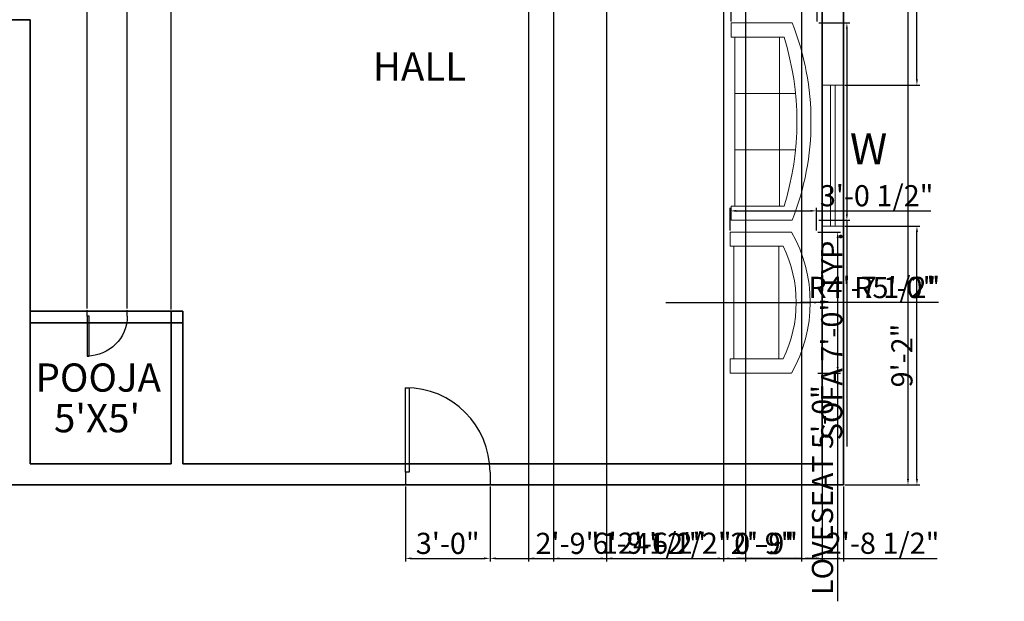
# Model space of a CAD drawing. Units: inches. Extents: x 3542 to 4275, y 1005 to 1722.
# Tile 2 of 6: x 3831 to 4250, y 1083 to 1330. Entities that reach past the tile are written whole.
import ezdxf

# ---------------------------------------------------------------- set-up
doc = ezdxf.new("R2010")
doc.units = ezdxf.units.IN
doc.layers.get('0').update_dxf_attribs({"color": 211})
for name, color, linetype, lineweight in [('A-ANNO-DIMS', 2, 'Continuous', 18), ('A-ANNO-TEXT', 7, 'Continuous', 18), ('A-AREA-IDEN', 7, 'Continuous', 25), ('A-DOOR', 3, 'Continuous', 25), ('A-FURN', 8, 'Continuous', 18), ('A-GLAZ', 4, 'Continuous', 18), ('wall', 7, 'Continuous', 35)]:
    doc.layers.add(name, color=color, linetype=linetype, lineweight=lineweight)
doc.styles.get("Standard").update_dxf_attribs({"font": 'arial.ttf'})
doc.dimstyles.new('ISO-25', dxfattribs={"dimtxt": 9, "dimasz": 2.5, "dimexe": 1.25, "dimexo": 0.625, "dimtad": 1, "dimdec": 1, "dimlunit": 4, "dimtxsty": 'Standard', "dimcen": 2.5, "dimadec": 0, "dimazin": 0, "dimtfac": 1, "dimtdec": 1, "dimtmove": 0, "dimatfit": 3, "dimfxl": 1, "dimarcsym": 0})

# ---------------------------------------------------------------- blocks, each defined once
blk = doc.blocks.new('*U2')
for p, q in [((0, 0), (0, -6)), ((40, 0), (40, -6))]:
    blk.add_line(p, q)
blk.add_lwpolyline([(0, 0), (0, 40), (1.75, 40), (1.75, 0)], close=True)
blk.add_arc((0, 0), 40, 0, 90)
blk = doc.blocks.new('Sofa - Roundback 7 ft.')
for p, q in [((-12.00002, -32.4421), (-12.00003, -6.5971)), ((11.99997, -32.4421), (11.99998, -6.5971)), ((-36.000027, -34), (-36.000027, -11.4696)), ((35.99998, -34), (35.99998, -11.4696)), ((-35.999844, -13.3819), (35.9998, -13.3819)), ((-36.000027, -32.4421), (35.99998, -32.4421))]:
    blk.add_line(p, q)
for points in [[(-36.000027, -34), (-42.000027, -34), (-42.000027, -8)], [(41.99998, -8), (41.99998, -34), (35.99998, -34)]]:
    blk.add_lwpolyline(points)
for centre, radius, start, end in [((0, -114.25), 114.25, 68.43141, 111.5686), ((-0.00001, -127.1968), 121.1968, 72.72033, 107.2797)]:
    blk.add_arc(centre, radius, start, end)
blk = doc.blocks.new('Sofa - Roundback Loveseat 5 ft.')
for p, q in [((0, -32.44198), (0, -5.99998)), ((-24, -33.99998), (-24, -11.46958)), ((24.00004, -33.99998), (24.00004, -11.46958)), ((-23.9998, -13.38178), (23.99986, -13.38178)), ((-24, -32.44198), (24.00004, -32.44198))]:
    blk.add_line(p, q)
for points in [[(-24, -33.99998), (-30, -33.99998), (-30, -7.99998)], [(30.00004, -7.99998), (30.00004, -33.99998), (24.00004, -33.99998)]]:
    blk.add_lwpolyline(points)
for centre, radius, start, end in [((0, -60.24998), 60.24998, 60.13715, 119.8628), ((0, -61.38438), 55.38444, 64.32083, 115.6792)]:
    blk.add_arc(centre, radius, start, end)
blk = doc.blocks.new('*D13')
at = {"layer": 'A-ANNO-DIMS', "color": 0, "lineweight": -2, "transparency": 16777216}
for p, q in [((4182.51, 1672.43), (4210.58, 1672.43)), ((4209.33, 1669.93), (4209.33, 1134.93)), ((4182.51, 1132.43), (4210.58, 1132.43))]:
    blk.add_line(p, q, dxfattribs=at)
at = {"layer": 'A-ANNO-DIMS', "color": 0, "transparency": 16777216}
for points in [[(4208.91, 1669.93), (4209.75, 1669.93), (4209.33, 1672.43)], [(4208.91, 1134.93), (4209.75, 1134.93), (4209.33, 1132.43)]]:
    blk.add_solid(points, dxfattribs=at)
at = {"layer": 'Defpoints', "color": 0, "transparency": 16777216}
for p in [(4181.89, 1672.43), (4181.89, 1132.43), (4209.33, 1132.43)]:
    blk.add_point(p, dxfattribs=at)
at = {"layer": 'A-ANNO-DIMS', "color": 0, "transparency": 16777216, "insert": (4204.13, 1402.43), "char_height": 9, "attachment_point": 5, "rotation": 90}
blk.add_mtext("45'", dxfattribs=at)
blk = doc.blocks.new('WIN-60IN')
for p, q in [((3.5, 60), (3.5, 0)), ((5.5, 60), (5.5, 0))]:
    blk.add_line(p, q)
blk.add_lwpolyline([(0, 60), (9, 60), (9, 0), (0, 0)], close=True)
blk = doc.blocks.new('*D23')
at = {"layer": 'A-ANNO-DIMS', "color": 0, "lineweight": -2, "transparency": 16777216}
for p, q in [((4171.36, 1329.06), (4184.59, 1329.06)), ((4183.34, 1326.56), (4183.34, 1247.56)), ((4171.36, 1245.06), (4184.59, 1245.06)), ((4183.34, 1245.06), (4183.34, 1148.77))]:
    blk.add_line(p, q, dxfattribs=at)
at = {"layer": 'A-ANNO-DIMS', "color": 0, "transparency": 16777216}
for points in [[(4182.92, 1326.56), (4183.76, 1326.56), (4183.34, 1329.06)], [(4182.92, 1247.56), (4183.76, 1247.56), (4183.34, 1245.06)]]:
    blk.add_solid(points, dxfattribs=at)
at = {"layer": 'Defpoints', "color": 0, "transparency": 16777216}
for p in [(4170.74, 1329.06), (4170.74, 1245.06), (4183.34, 1245.06)]:
    blk.add_point(p, dxfattribs=at)
at = {"layer": 'A-ANNO-DIMS', "color": 0, "transparency": 16777216, "insert": (4178.06, 1195.66), "char_height": 9, "attachment_point": 5, "rotation": 90}
blk.add_mtext('SOFA 7\'-0" TYP.', dxfattribs=at)
blk = doc.blocks.new('*D24')
at = {"layer": 'A-ANNO-DIMS', "color": 0, "lineweight": -2, "transparency": 16777216}
for p, q in [((4134.07, 1329.69), (4134.07, 1342.91)), ((4136.57, 1341.66), (4168.24, 1341.66)), ((4170.74, 1329.69), (4170.74, 1342.91)), ((4170.74, 1341.66), (4250.31, 1341.66))]:
    blk.add_line(p, q, dxfattribs=at)
at = {"layer": 'A-ANNO-DIMS', "color": 0, "transparency": 16777216}
for points in [[(4136.57, 1342.08), (4136.57, 1341.24), (4134.07, 1341.66)], [(4168.24, 1342.08), (4168.24, 1341.24), (4170.74, 1341.66)]]:
    blk.add_solid(points, dxfattribs=at)
at = {"layer": 'Defpoints', "color": 0, "transparency": 16777216}
for p in [(4170.74, 1341.66), (4134.07, 1329.06), (4170.74, 1329.06)]:
    blk.add_point(p, dxfattribs=at)
at = {"layer": 'A-ANNO-DIMS', "color": 0, "transparency": 16777216, "insert": (4211.78, 1346.94), "char_height": 9, "attachment_point": 5}
blk.add_mtext('3\'-0 1/2" TYP.', dxfattribs=at)
blk = doc.blocks.new('*D29')
at = {"layer": 'A-ANNO-DIMS', "color": 0, "lineweight": -2, "transparency": 16777216}
for p, q in [((4171.04, 1240.07), (4180.66, 1240.07)), ((4179.41, 1237.57), (4179.41, 1182.57)), ((4171.04, 1180.07), (4180.66, 1180.07)), ((4179.41, 1180.07), (4179.41, 1082.92))]:
    blk.add_line(p, q, dxfattribs=at)
at = {"layer": 'A-ANNO-DIMS', "color": 0, "transparency": 16777216}
for points in [[(4179, 1237.57), (4179.83, 1237.57), (4179.41, 1240.07)], [(4179, 1182.57), (4179.83, 1182.57), (4179.41, 1180.07)]]:
    blk.add_solid(points, dxfattribs=at)
at = {"layer": 'Defpoints', "color": 0, "transparency": 16777216}
for p in [(4170.41, 1240.07), (4170.41, 1180.07), (4179.41, 1180.07)]:
    blk.add_point(p, dxfattribs=at)
at = {"layer": 'A-ANNO-DIMS', "color": 0, "transparency": 16777216, "insert": (4174.13, 1130.24), "char_height": 9, "attachment_point": 5, "rotation": 90}
blk.add_mtext('LOVESEAT 5\'-0"', dxfattribs=at)
blk = doc.blocks.new('*D30')
at = {"layer": 'A-ANNO-DIMS', "color": 0, "lineweight": -2, "transparency": 16777216}
for p, q in [((4133.75, 1240.69), (4133.75, 1250.32)), ((4136.25, 1249.07), (4167.91, 1249.07)), ((4170.41, 1240.69), (4170.41, 1250.32)), ((4170.41, 1249.07), (4219.05, 1249.07))]:
    blk.add_line(p, q, dxfattribs=at)
at = {"layer": 'A-ANNO-DIMS', "color": 0, "transparency": 16777216}
for points in [[(4136.25, 1249.49), (4136.25, 1248.65), (4133.75, 1249.07)], [(4167.91, 1249.49), (4167.91, 1248.65), (4170.41, 1249.07)]]:
    blk.add_solid(points, dxfattribs=at)
at = {"layer": 'Defpoints', "color": 0, "transparency": 16777216}
for p in [(4170.41, 1249.07), (4133.75, 1240.07), (4170.41, 1240.07)]:
    blk.add_point(p, dxfattribs=at)
at = {"layer": 'A-ANNO-DIMS', "color": 0, "transparency": 16777216, "insert": (4195.98, 1254.35), "char_height": 9, "attachment_point": 5}
blk.add_mtext('3\'-0 1/2"', dxfattribs=at)
blk = doc.blocks.new('*D38')
at = {"layer": 'A-ANNO-DIMS', "color": 0, "lineweight": -2, "transparency": 16777216}
for p, q in [((4182.51, 1242.58), (4214.39, 1242.58)), ((4213.14, 1134.93), (4213.14, 1240.08)), ((4182.51, 1132.43), (4214.39, 1132.43))]:
    blk.add_line(p, q, dxfattribs=at)
at = {"layer": 'A-ANNO-DIMS', "color": 0, "transparency": 16777216}
for points in [[(4212.72, 1240.08), (4213.56, 1240.08), (4213.14, 1242.58)], [(4212.72, 1134.93), (4213.56, 1134.93), (4213.14, 1132.43)]]:
    blk.add_solid(points, dxfattribs=at)
at = {"layer": 'Defpoints', "color": 0, "transparency": 16777216}
for p in [(4181.89, 1242.58), (4213.14, 1242.58), (4181.89, 1132.43)]:
    blk.add_point(p, dxfattribs=at)
at = {"layer": 'A-ANNO-DIMS', "color": 0, "transparency": 16777216, "insert": (4207.92, 1187.5), "char_height": 9, "attachment_point": 5, "rotation": 90}
blk.add_mtext('9\'-2"', dxfattribs=at)
blk = doc.blocks.new('*D39')
at = {"layer": 'A-ANNO-DIMS', "color": 0, "lineweight": -2, "transparency": 16777216}
for p, q in [((4182.51, 1503.8), (4214.39, 1503.8)), ((4213.14, 1305.08), (4213.14, 1501.3)), ((4182.51, 1302.58), (4214.39, 1302.58))]:
    blk.add_line(p, q, dxfattribs=at)
at = {"layer": 'A-ANNO-DIMS', "color": 0, "transparency": 16777216}
for points in [[(4212.72, 1501.3), (4213.56, 1501.3), (4213.14, 1503.8)], [(4212.72, 1305.08), (4213.56, 1305.08), (4213.14, 1302.58)]]:
    blk.add_solid(points, dxfattribs=at)
at = {"layer": 'Defpoints', "color": 0, "transparency": 16777216}
for p in [(4181.89, 1503.8), (4213.14, 1503.8), (4181.89, 1302.58)]:
    blk.add_point(p, dxfattribs=at)
at = {"layer": 'A-ANNO-DIMS', "color": 0, "transparency": 16777216, "insert": (4207.92, 1403.19), "char_height": 9, "attachment_point": 5, "rotation": 90}
blk.add_mtext('16\'-9"', dxfattribs=at)
blk = doc.blocks.new('*D40')
at = {"layer": 'A-ANNO-DIMS', "color": 0, "lineweight": -2, "transparency": 16777216}
for p, q in [((4031.51, 1131.8), (4031.51, 1099.93)), ((4181.89, 1131.8), (4181.89, 1099.93)), ((4034.01, 1101.18), (4179.39, 1101.18))]:
    blk.add_line(p, q, dxfattribs=at)
at = {"layer": 'A-ANNO-DIMS', "color": 0, "transparency": 16777216}
for points in [[(4034.01, 1101.59), (4034.01, 1100.76), (4031.51, 1101.18)], [(4179.39, 1101.59), (4179.39, 1100.76), (4181.89, 1101.18)]]:
    blk.add_solid(points, dxfattribs=at)
at = {"layer": 'Defpoints', "color": 0, "transparency": 16777216}
for p in [(4031.51, 1132.43), (4181.89, 1132.43), (4181.89, 1101.18)]:
    blk.add_point(p, dxfattribs=at)
at = {"layer": 'A-ANNO-DIMS', "color": 0, "transparency": 16777216, "insert": (4106.7, 1106.46), "char_height": 9, "attachment_point": 5}
blk.add_mtext('12\'-6 1/2"', dxfattribs=at)
blk = doc.blocks.new('*D41')
at = {"layer": 'A-ANNO-DIMS', "color": 0, "lineweight": -2, "transparency": 16777216}
for p, q in [((3995.51, 1131.8), (3995.51, 1099.93)), ((4031.51, 1131.8), (4031.51, 1099.93)), ((3998.01, 1101.18), (4029.01, 1101.18))]:
    blk.add_line(p, q, dxfattribs=at)
at = {"layer": 'A-ANNO-DIMS', "color": 0, "transparency": 16777216}
for points in [[(3998.01, 1101.59), (3998.01, 1100.76), (3995.51, 1101.18)], [(4029.01, 1101.59), (4029.01, 1100.76), (4031.51, 1101.18)]]:
    blk.add_solid(points, dxfattribs=at)
at = {"layer": 'Defpoints', "color": 0, "transparency": 16777216}
for p in [(3995.51, 1132.43), (4031.51, 1132.43), (4031.51, 1101.18)]:
    blk.add_point(p, dxfattribs=at)
at = {"layer": 'A-ANNO-DIMS', "color": 0, "transparency": 16777216, "insert": (4013.51, 1106.4), "char_height": 9, "attachment_point": 5}
blk.add_mtext('3\'-0"', dxfattribs=at)
blk = doc.blocks.new('*D49')
at = {"layer": 'A-ANNO-DIMS', "color": 0, "lineweight": -2, "transparency": 16777216}
for p, q in [((4058.5, 1442.8), (4058.5, 1099.93)), ((4140.16, 1442.8), (4140.16, 1099.93)), ((4061, 1101.18), (4137.66, 1101.18))]:
    blk.add_line(p, q, dxfattribs=at)
at = {"layer": 'A-ANNO-DIMS', "color": 0, "transparency": 16777216}
for points in [[(4061, 1101.59), (4061, 1100.76), (4058.5, 1101.18)], [(4137.66, 1101.59), (4137.66, 1100.76), (4140.16, 1101.18)]]:
    blk.add_solid(points, dxfattribs=at)
at = {"layer": 'Defpoints', "color": 0, "transparency": 16777216}
for p in [(4058.5, 1443.43), (4140.16, 1443.43), (4140.16, 1101.18)]:
    blk.add_point(p, dxfattribs=at)
at = {"layer": 'A-ANNO-DIMS', "color": 0, "transparency": 16777216, "insert": (4099.33, 1106.46), "char_height": 9, "attachment_point": 5}
blk.add_mtext('6\'-9 1/2"', dxfattribs=at)
blk = doc.blocks.new('*D50')
at = {"layer": 'A-ANNO-DIMS', "color": 0, "lineweight": -2, "transparency": 16777216}
for p, q in [((4140.16, 1442.8), (4140.16, 1099.93)), ((4172.89, 1442.8), (4172.89, 1099.93)), ((4142.66, 1101.18), (4170.39, 1101.18)), ((4172.89, 1101.18), (4221.69, 1101.18))]:
    blk.add_line(p, q, dxfattribs=at)
at = {"layer": 'A-ANNO-DIMS', "color": 0, "transparency": 16777216}
for points in [[(4142.66, 1101.59), (4142.66, 1100.76), (4140.16, 1101.18)], [(4170.39, 1101.59), (4170.39, 1100.76), (4172.89, 1101.18)]]:
    blk.add_solid(points, dxfattribs=at)
at = {"layer": 'Defpoints', "color": 0, "transparency": 16777216}
for p in [(4140.16, 1443.43), (4172.89, 1443.43), (4172.89, 1101.18)]:
    blk.add_point(p, dxfattribs=at)
at = {"layer": 'A-ANNO-DIMS', "color": 0, "transparency": 16777216, "insert": (4198.54, 1106.46), "char_height": 9, "attachment_point": 5}
blk.add_mtext('2\'-8 1/2"', dxfattribs=at)
blk = doc.blocks.new('*D51')
at = {"layer": 'A-ANNO-DIMS', "color": 0, "lineweight": -2, "transparency": 16777216}
for p, q in [((4047.82, 1510.06), (4047.82, 1099.93)), ((4081.03, 1510.06), (4081.03, 1099.93)), ((4050.32, 1101.18), (4078.53, 1101.18))]:
    blk.add_line(p, q, dxfattribs=at)
at = {"layer": 'A-ANNO-DIMS', "color": 0, "transparency": 16777216}
for points in [[(4050.32, 1101.59), (4050.32, 1100.76), (4047.82, 1101.18)], [(4078.53, 1101.59), (4078.53, 1100.76), (4081.03, 1101.18)]]:
    blk.add_solid(points, dxfattribs=at)
at = {"layer": 'Defpoints', "color": 0, "transparency": 16777216}
for p in [(4047.82, 1510.69), (4081.03, 1510.69), (4081.03, 1101.18)]:
    blk.add_point(p, dxfattribs=at)
at = {"layer": 'A-ANNO-DIMS', "color": 0, "transparency": 16777216, "insert": (4064.42, 1106.4), "char_height": 9, "attachment_point": 5}
blk.add_mtext('2\'-9"', dxfattribs=at)
blk = doc.blocks.new('*D52')
at = {"layer": 'A-ANNO-DIMS', "color": 0, "lineweight": -2, "transparency": 16777216}
for p, q in [((4081.03, 1510.06), (4081.03, 1099.93)), ((4130.83, 1463.03), (4130.83, 1099.93)), ((4083.53, 1101.18), (4128.33, 1101.18))]:
    blk.add_line(p, q, dxfattribs=at)
at = {"layer": 'A-ANNO-DIMS', "color": 0, "transparency": 16777216}
for points in [[(4083.53, 1101.59), (4083.53, 1100.76), (4081.03, 1101.18)], [(4128.33, 1101.59), (4128.33, 1100.76), (4130.83, 1101.18)]]:
    blk.add_solid(points, dxfattribs=at)
at = {"layer": 'Defpoints', "color": 0, "transparency": 16777216}
for p in [(4081.03, 1510.69), (4130.83, 1463.65), (4130.83, 1101.18)]:
    blk.add_point(p, dxfattribs=at)
at = {"layer": 'A-ANNO-DIMS', "color": 0, "transparency": 16777216, "insert": (4105.93, 1106.32), "char_height": 9, "attachment_point": 5}
blk.add_mtext('4\'-2"', dxfattribs=at)
blk = doc.blocks.new('*D53')
at = {"layer": 'A-ANNO-DIMS', "color": 0, "lineweight": -2, "transparency": 16777216}
for p, q in [((4130.83, 1463.03), (4130.83, 1099.93)), ((4164.03, 1463.03), (4164.03, 1099.93)), ((4133.33, 1101.18), (4161.53, 1101.18))]:
    blk.add_line(p, q, dxfattribs=at)
at = {"layer": 'A-ANNO-DIMS', "color": 0, "transparency": 16777216}
for points in [[(4133.33, 1101.59), (4133.33, 1100.76), (4130.83, 1101.18)], [(4161.53, 1101.59), (4161.53, 1100.76), (4164.03, 1101.18)]]:
    blk.add_solid(points, dxfattribs=at)
at = {"layer": 'Defpoints', "color": 0, "transparency": 16777216}
for p in [(4130.83, 1463.65), (4164.03, 1463.65), (4164.03, 1101.18)]:
    blk.add_point(p, dxfattribs=at)
at = {"layer": 'A-ANNO-DIMS', "color": 0, "transparency": 16777216, "insert": (4147.43, 1106.4), "char_height": 9, "attachment_point": 5}
blk.add_mtext('2\'-9"', dxfattribs=at)
blk = doc.blocks.new('*D57')
at = {"layer": 'A-ANNO-DIMS', "color": 0, "lineweight": -2, "transparency": 16777216}
for p, q in [((4164.03, 1463.03), (4164.03, 1099.93)), ((4172.89, 1447.8), (4172.89, 1099.93)), ((4164.03, 1101.18), (4136.35, 1101.18)), ((4170.39, 1101.18), (4166.53, 1101.18))]:
    blk.add_line(p, q, dxfattribs=at)
at = {"layer": 'A-ANNO-DIMS', "color": 0, "transparency": 16777216}
for points in [[(4166.53, 1101.59), (4166.53, 1100.76), (4164.03, 1101.18)], [(4170.39, 1101.59), (4170.39, 1100.76), (4172.89, 1101.18)]]:
    blk.add_solid(points, dxfattribs=at)
at = {"layer": 'Defpoints', "color": 0, "transparency": 16777216}
for p in [(4164.03, 1463.65), (4172.89, 1448.43), (4164.03, 1101.18)]:
    blk.add_point(p, dxfattribs=at)
at = {"layer": 'A-ANNO-DIMS', "color": 0, "transparency": 16777216, "insert": (4148.94, 1106.4), "char_height": 9, "attachment_point": 5}
blk.add_mtext('0\'-9"', dxfattribs=at)
blk = doc.blocks.new('*D60')
at = {"layer": 'A-ANNO-DIMS', "color": 0, "lineweight": -2, "transparency": 16777216}
for p, q in [((3860.16, 1207.47), (3860.16, 1704.93)), ((3877.16, 1207.47), (3877.16, 1704.93)), ((3860.16, 1703.68), (3833.33, 1703.68)), ((3874.66, 1703.68), (3862.66, 1703.68))]:
    blk.add_line(p, q, dxfattribs=at)
at = {"layer": 'A-ANNO-DIMS', "color": 0, "transparency": 16777216}
for points in [[(3862.66, 1704.09), (3862.66, 1703.26), (3860.16, 1703.68)], [(3874.66, 1704.09), (3874.66, 1703.26), (3877.16, 1703.68)]]:
    blk.add_solid(points, dxfattribs=at)
at = {"layer": 'Defpoints', "color": 0, "transparency": 16777216}
for p in [(3860.16, 1703.68), (3860.16, 1206.85), (3877.16, 1206.85)]:
    blk.add_point(p, dxfattribs=at)
at = {"layer": 'A-ANNO-DIMS', "color": 0, "transparency": 16777216, "insert": (3845.5, 1708.9), "char_height": 9, "attachment_point": 5}
blk.add_mtext('1\'-5"', dxfattribs=at)
blk = doc.blocks.new('*D61')
at = {"layer": 'A-ANNO-DIMS', "color": 0, "lineweight": -2, "transparency": 16777216}
for p, q in [((3877.16, 1207.47), (3877.16, 1704.93)), ((3895.89, 1207.05), (3895.89, 1704.93)), ((3877.16, 1703.68), (3829.36, 1703.68)), ((3893.39, 1703.68), (3879.66, 1703.68))]:
    blk.add_line(p, q, dxfattribs=at)
at = {"layer": 'A-ANNO-DIMS', "color": 0, "transparency": 16777216}
for points in [[(3879.66, 1704.09), (3879.66, 1703.26), (3877.16, 1703.68)], [(3893.39, 1704.09), (3893.39, 1703.26), (3895.89, 1703.68)]]:
    blk.add_solid(points, dxfattribs=at)
at = {"layer": 'Defpoints', "color": 0, "transparency": 16777216}
for p in [(3877.16, 1703.68), (3877.16, 1206.85), (3895.89, 1206.43)]:
    blk.add_point(p, dxfattribs=at)
at = {"layer": 'A-ANNO-DIMS', "color": 0, "transparency": 16777216, "insert": (3852.01, 1708.96), "char_height": 9, "attachment_point": 5}
blk.add_mtext('1\'-6 1/2"', dxfattribs=at)
blk = doc.blocks.new('*D76')
at = {"layer": 'A-ANNO-DIMS', "color": 0, "lineweight": -2, "transparency": 16777216}
for p, q in [((4107.5, 1210.07), (4167.75, 1210.07)), ((4220.79, 1210.07), (4170.25, 1210.07))]:
    blk.add_line(p, q, dxfattribs=at)
at = {"layer": 'A-ANNO-DIMS', "color": 0, "transparency": 16777216}
blk.add_solid([(4170.25, 1210.49), (4170.25, 1209.65), (4167.75, 1210.07)], dxfattribs=at)
at = {"layer": 'Defpoints', "color": 0, "transparency": 16777216}
for p in [(4107.5, 1210.07), (4167.75, 1210.07)]:
    blk.add_point(p, dxfattribs=at)
at = {"layer": 'A-ANNO-DIMS', "color": 0, "transparency": 16777216, "insert": (4203.9, 1215.29), "char_height": 9, "attachment_point": 5, "rotation": 0.0004}
blk.add_mtext('R5\'-0"', dxfattribs=at)
blk = doc.blocks.new('*D77')
at = {"layer": 'A-ANNO-DIMS', "color": 0, "lineweight": -2, "transparency": 16777216}
for p, q in [((4106.36, 1210.07), (4161.75, 1210.07)), ((4222.36, 1210.07), (4164.25, 1210.07))]:
    blk.add_line(p, q, dxfattribs=at)
at = {"layer": 'A-ANNO-DIMS', "color": 0, "transparency": 16777216}
blk.add_solid([(4164.25, 1210.49), (4164.25, 1209.65), (4161.75, 1210.07)], dxfattribs=at)
at = {"layer": 'Defpoints', "color": 0, "transparency": 16777216}
for p in [(4106.36, 1210.07), (4161.75, 1210.07)]:
    blk.add_point(p, dxfattribs=at)
at = {"layer": 'A-ANNO-DIMS', "color": 0, "transparency": 16777216, "insert": (4194.98, 1215.35), "char_height": 9, "attachment_point": 5, "rotation": 0.0004}
blk.add_mtext('R4\'-7 1/2"', dxfattribs=at)

msp = doc.modelspace()

# ---------------------------------------------------------------- linework, layer by layer
at = {"layer": 'wall'}
for p, q in [((4181.89, 1672.43), (4181.89, 1132.43)), ((4172.89, 1443.43), (4172.89, 1141.43)), ((3739.89, 1330.43), (3835.89, 1330.43)), ((3835.89, 1141.43), (3835.89, 1330.43)), ((3900.89, 1206.43), (3835.89, 1206.43)), ((3895.89, 1141.43), (3895.89, 1206.43)), ((3900.89, 1141.43), (3900.89, 1206.43)), ((3900.89, 1201.43), (3835.89, 1201.43)), ((3895.89, 1141.43), (3835.89, 1141.43)), ((3895.89, 1141.43), (3835.89, 1141.43)), ((4172.89, 1141.43), (3900.89, 1141.43)), ((4015.89, 1141.43), (3900.89, 1141.43)), ((4181.89, 1132.43), (3641.89, 1132.43))]:
    msp.add_line(p, q, dxfattribs=at)

# ---------------------------------------------------------------- block references
at = {"layer": 'A-DOOR', "xscale": -0.425, "yscale": 0.425, "zscale": 0.425, "rotation": 180}
msp.add_blockref('*U2', (3860.16, 1204.3), dxfattribs=at)
at = {"layer": 'A-DOOR', "xscale": 0.9, "yscale": 0.9, "zscale": 0.9}
msp.add_blockref('*U2', (3995.51, 1137.83), dxfattribs=at)
at = {"layer": 'A-FURN', "rotation": 270}
for name, p in [('Sofa - Roundback 7 ft.', (4168.07, 1287.06)), ('Sofa - Roundback Loveseat 5 ft.', (4167.75, 1210.07))]:
    msp.add_blockref(name, p, dxfattribs=at)
at = {"layer": 'A-GLAZ'}
msp.add_blockref('WIN-60IN', (4172.89, 1242.58), dxfattribs=at)

# ---------------------------------------------------------------- texts
at = {"layer": 'A-ANNO-TEXT'}
msp.add_text('W', height=13.28, dxfattribs=at).set_placement((4184.61, 1268.84))
at = {"layer": 'A-AREA-IDEN'}
for s, p in [('HALL', (3981.7, 1304.48)), ('POOJA', (3838.16, 1172.14)), ("5'X5'", (3846, 1154.84))]:
    msp.add_text(s, height=12, dxfattribs=at).set_placement(p)

# ---------------------------------------------------------------- dimensions: what is measured, and where the dimension line sits
at = {"layer": 'A-ANNO-DIMS'}
for base, p1, p2, picture, middle in [((3877.16, 1703.68), (3895.89, 1206.43), (3877.16, 1206.85), '*D61', (3852.01, 1708.96)), ((3860.16, 1703.68), (3877.16, 1206.85), (3860.16, 1206.85), '*D60', (3845.5, 1708.9)), ((4081.03, 1101.18), (4047.82, 1510.69), (4081.03, 1510.69), '*D51', (4064.42, 1106.4)), ((4130.83, 1101.18), (4081.03, 1510.69), (4130.83, 1463.65), '*D52', (4105.93, 1106.32)), ((4164.03, 1101.18), (4130.83, 1463.65), (4164.03, 1463.65), '*D53', (4147.43, 1106.4)), ((4164.03, 1101.18), (4172.89, 1448.43), (4164.03, 1463.65), '*D57', (4148.94, 1106.4)), ((4140.16, 1101.18), (4058.5, 1443.43), (4140.16, 1443.43), '*D49', (4099.33, 1106.46)), ((4172.89, 1101.18), (4140.16, 1443.43), (4172.89, 1443.43), '*D50', (4198.54, 1106.46)), ((4170.41, 1249.07), (4133.75, 1240.07), (4170.41, 1240.07), '*D30', (4195.98, 1254.35)), ((4031.51, 1101.18), (3995.51, 1132.43), (4031.51, 1132.43), '*D41', (4013.51, 1106.4)), ((4181.89, 1101.18), (4031.51, 1132.43), (4181.89, 1132.43), '*D40', (4106.7, 1106.46))]:
    dim = msp.add_linear_dim(base=base, p1=p1, p2=p2, dimstyle='ISO-25', override={"dimdec": 1, "dimlfac": 1, "dimrnd": 0, "dimzin": 1, "dimdsep": 46, "dimlunit": 4, "dimfrac": 2}, dxfattribs=at)
    dim.commit()
    dim.dimension.update_dxf_attribs({"geometry": picture, "text_midpoint": middle})
for base, p1, p2, override, picture, middle in [((4209.33, 1132.43), (4181.89, 1672.43), (4181.89, 1132.43), {"dimclrd": 0, "dimclre": 0, "dimclrt": 0}, '*D13', (4204.13, 1402.43)), ((4213.14, 1503.8), (4181.89, 1302.58), (4181.89, 1503.8), {"dimdec": 1, "dimlfac": 1, "dimrnd": 0, "dimzin": 1, "dimdsep": 46, "dimlunit": 4, "dimfrac": 2}, '*D39', (4207.92, 1403.19)), ((4213.1394, 1242.5773), (4181.8894, 1132.4279), (4181.8894, 1242.5773), {"dimdec": 1, "dimlfac": 1, "dimrnd": 0, "dimzin": 1, "dimdsep": 46, "dimlunit": 4, "dimfrac": 2}, '*D38', (4207.9192, 1187.5026))]:
    dim = msp.add_linear_dim(base=base, p1=p1, p2=p2, angle=90, dimstyle='ISO-25', override=override, dxfattribs=at)
    dim.commit()
    dim.dimension.update_dxf_attribs({"geometry": picture, "text_midpoint": middle})
dim = msp.add_linear_dim(base=(4170.74, 1341.66), p1=(4134.07, 1329.06), p2=(4170.74, 1329.06), text='<> TYP.', dimstyle='ISO-25', override={"dimdec": 1, "dimlfac": 1, "dimrnd": 0, "dimzin": 1, "dimdsep": 46, "dimlunit": 4, "dimfrac": 2}, dxfattribs=at)
dim.commit()
dim.dimension.update_dxf_attribs({"geometry": '*D24', "text_midpoint": (4211.78, 1346.94)})
for base, p1, p2, text, picture, middle in [((4183.34, 1245.06), (4170.74, 1329.06), (4170.74, 1245.06), 'SOFA <> TYP.', '*D23', (4178.06, 1195.66)), ((4179.41, 1180.07), (4170.41, 1240.07), (4170.41, 1180.07), 'LOVESEAT <>', '*D29', (4174.13, 1130.24))]:
    dim = msp.add_linear_dim(base=base, p1=p1, p2=p2, angle=270, text=text, dimstyle='ISO-25', override={"dimdec": 1, "dimlfac": 1, "dimrnd": 0, "dimzin": 1, "dimdsep": 46, "dimlunit": 4, "dimfrac": 2}, dxfattribs=at)
    dim.commit()
    dim.dimension.update_dxf_attribs({"geometry": picture, "text_midpoint": middle})
for center, mpoint, picture, middle in [((4106.36, 1210.07), (4161.75, 1210.07), '*D77', (4194.98, 1210.07)), ((4107.49714, 1210.06958), (4167.74712, 1210.07), '*D76', (4203.89711, 1210.07025))]:
    dim = msp.add_radius_dim(center=center, mpoint=mpoint, dimstyle='ISO-25', override={"dimdec": 1, "dimlfac": 1, "dimrnd": 0, "dimzin": 1, "dimdsep": 46, "dimlunit": 4, "dimfrac": 2}, dxfattribs=at)
    dim.commit()
    dim.dimension.update_dxf_attribs({"geometry": picture, "text_midpoint": middle, "dimtype": 164})

doc.saveas('drawing.dxf')
